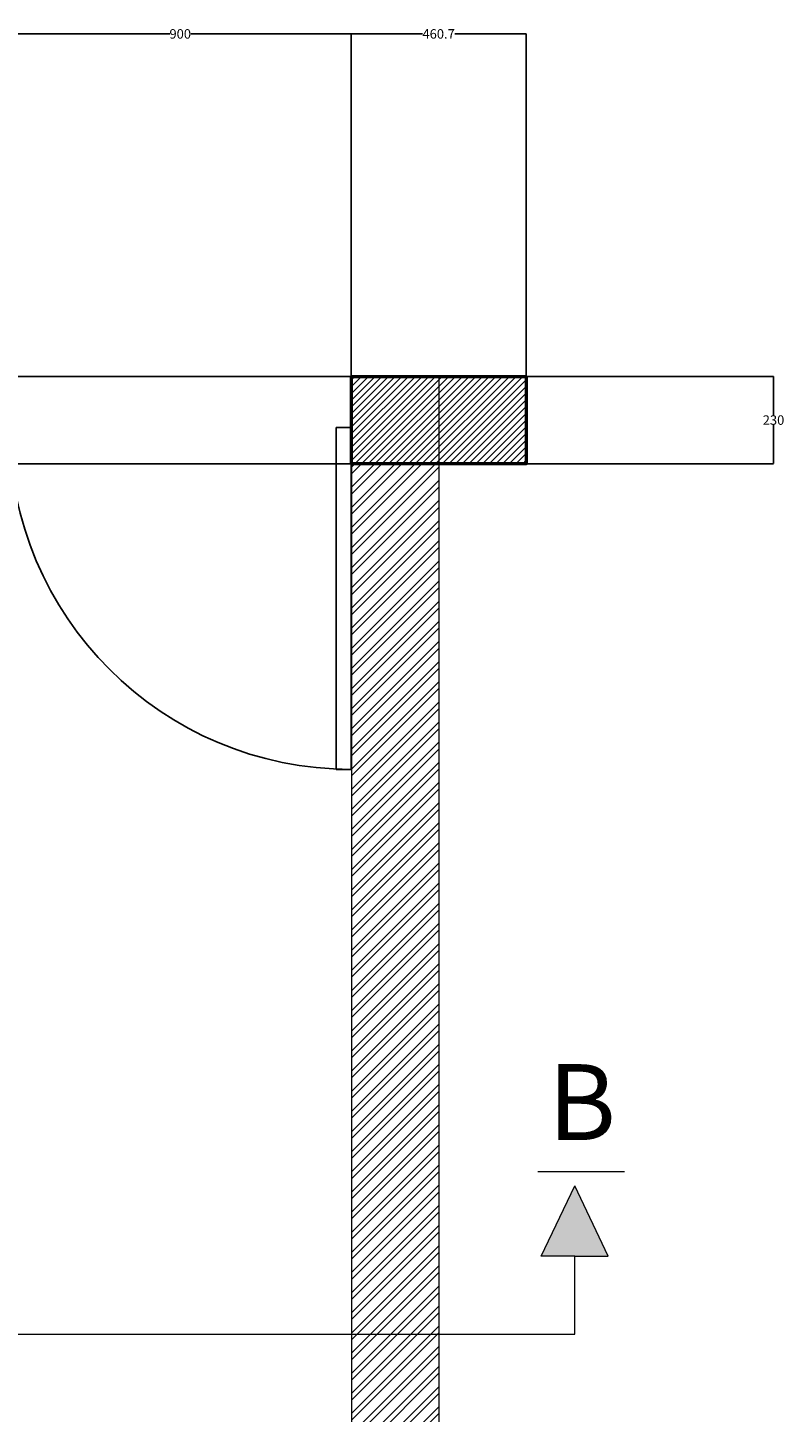
# Model space of a CAD drawing. Units: millimetres. Extents: x 1944 to 29915, y -10550 to 5909.
# Tile 9 of 24: x 9044 to 11036, y 2263 to 5909. Entities that reach past the tile are written whole.
import ezdxf

# ---------------------------------------------------------------- set-up
doc = ezdxf.new("R2010")
doc.units = ezdxf.units.MM
doc.header["$MEASUREMENT"] = 0
for name, color, linetype, lineweight in [('A-ANNO-DIMS', 2, 'Continuous', 18), ('A-ANNO-SYMB', 2, 'Continuous', 18), ('A-ANNO-TEXT', 7, 'Continuous', 25), ('A-DOOR', 4, 'Continuous', 25), ('A-FLOR-FIXT', 9, 'Continuous', 18), ('A-WALL', 7, 'Continuous', 50), ('A-WALL-PATT', 8, 'Continuous', 18)]:
    doc.layers.add(name, color=color, linetype=linetype, lineweight=lineweight)
doc.styles.get("Standard").update_dxf_attribs({"font": 'arial.ttf'})
doc.dimstyles.get("Standard").update_dxf_attribs({"dimtxt": 25, "dimasz": 0.18, "dimexe": 0.18, "dimexo": 0.0625, "dimgap": 0.09, "dimtad": 0, "dimtih": 1, "dimtoh": 1, "dimdec": 0, "dimzin": 0, "dimdsep": 46, "dimtxsty": 'Standard', "dimcen": 0.09, "dimadec": 0, "dimazin": 0, "dimtfac": 1, "dimtdec": 0, "dimtofl": 0, "dimtmove": 0, "dimatfit": 3, "dimfxl": 1, "dimtolj": 1, "dimtzin": 0, "dimarcsym": 0})

# ---------------------------------------------------------------- blocks, each defined once
blk = doc.blocks.new('*U2')
for p, q in [((0, 0), (0, -6)), ((40, 0), (40, -6))]:
    blk.add_line(p, q)
blk.add_lwpolyline([(0, 0), (0, 40), (1.75, 40), (1.75, 0)], close=True)
blk.add_arc((0, 0), 40, 0, 90)
blk = doc.blocks.new('*D47')
at = {"layer": 'A-ANNO-DIMS', "color": 0, "lineweight": -2, "transparency": 16777216}
for p, q in [((8995.2, 4990.9), (8995.2, 5892.9)), ((8995.4, 5892.8), (9417.6, 5892.8)), ((9895, 5892.8), (9472.9, 5892.8)), ((9895.2, 4990.9), (9895.2, 5892.9))]:
    blk.add_line(p, q, dxfattribs=at)
at = {"layer": 'A-ANNO-DIMS', "color": 0, "transparency": 16777216}
for points in [[(8995.4, 5892.8), (8995.4, 5892.7), (8995.2, 5892.8)], [(9895, 5892.8), (9895, 5892.7), (9895.2, 5892.8)]]:
    blk.add_solid(points, dxfattribs=at)
at = {"layer": 'Defpoints', "color": 0, "transparency": 16777216}
for p in [(9895.2, 5892.8), (8995.2, 4990.8), (9895.2, 4990.8)]:
    blk.add_point(p, dxfattribs=at)
at = {"layer": 'A-ANNO-DIMS', "color": 0, "transparency": 16777216, "insert": (9445.2, 5892.8), "char_height": 25, "attachment_point": 5}
blk.add_mtext('\\A1;900', dxfattribs=at)
blk = doc.blocks.new('*D48')
at = {"layer": 'A-ANNO-DIMS', "color": 0, "lineweight": -2, "transparency": 16777216}
for p, q in [((9895.2, 4990.9), (9895.2, 5892.9)), ((9895.4, 5892.8), (10082.8, 5892.8)), ((10355.8, 5892.8), (10168.4, 5892.8)), ((10355.9, 4990.9), (10355.9, 5892.9))]:
    blk.add_line(p, q, dxfattribs=at)
at = {"layer": 'A-ANNO-DIMS', "color": 0, "transparency": 16777216}
for points in [[(9895.4, 5892.8), (9895.4, 5892.7), (9895.2, 5892.8)], [(10355.8, 5892.8), (10355.8, 5892.7), (10355.9, 5892.8)]]:
    blk.add_solid(points, dxfattribs=at)
at = {"layer": 'Defpoints', "color": 0, "transparency": 16777216}
for p in [(10355.9, 5892.8), (9895.2, 4990.8), (10355.9, 4990.8)]:
    blk.add_point(p, dxfattribs=at)
at = {"layer": 'A-ANNO-DIMS', "color": 0, "transparency": 16777216, "insert": (10125.6, 5892.8), "char_height": 25, "attachment_point": 5}
blk.add_mtext('\\A1;460.7', dxfattribs=at)
blk = doc.blocks.new('*D55')
at = {"layer": 'A-ANNO-DIMS', "color": 0, "lineweight": -2, "transparency": 16777216}
for p, q in [((8995.3, 4990.8), (11007.7, 4990.8)), ((11007.5, 4990.7), (11007.5, 4888.7)), ((11007.5, 4761), (11007.5, 4863)), ((8995.3, 4760.8), (11007.7, 4760.8))]:
    blk.add_line(p, q, dxfattribs=at)
at = {"layer": 'A-ANNO-DIMS', "color": 0, "transparency": 16777216}
for points in [[(11007.5, 4990.7), (11007.5, 4990.7), (11007.5, 4990.8)], [(11007.5, 4761), (11007.5, 4761), (11007.5, 4760.8)]]:
    blk.add_solid(points, dxfattribs=at)
at = {"layer": 'Defpoints', "color": 0, "transparency": 16777216}
for p in [(8995.2, 4990.8), (8995.2, 4760.8), (11007.5, 4760.8)]:
    blk.add_point(p, dxfattribs=at)
at = {"layer": 'A-ANNO-DIMS', "color": 0, "transparency": 16777216, "insert": (11007.5, 4875.8), "char_height": 25, "attachment_point": 5}
blk.add_mtext('\\A1;230', dxfattribs=at)

msp = doc.modelspace()

# ---------------------------------------------------------------- hatches: boundary and pattern name
at = {"layer": 'A-ANNO-SYMB'}
h = msp.add_hatch(color=256, dxfattribs=at)
h.dxf.hatch_style = 1
h.paths.add_polyline_path([(10483.966, 2859.206), (10395.936, 2673.669), (10483.966, 2673.669), (10571.997, 2673.669)])
at = {"layer": 'A-WALL-PATT'}
h = msp.add_hatch(dxfattribs=at)
h.set_pattern_fill('ANSI31', color=256, scale=100)
h.paths.add_polyline_path([(9895.942, 4990.837), (9895.942, 4760.837), (10355.942, 4760.837), (10355.942, 4990.837)])
h = msp.add_hatch(dxfattribs=at)
h.set_pattern_fill('ANSI32', color=256, scale=100)
h.paths.add_polyline_path([(9895.942, 490.837), (10125.942, 490.837), (10125.942, 4760.837), (9895.942, 4760.837)])

# ---------------------------------------------------------------- linework, layer by layer
at = {"layer": 'A-ANNO-SYMB'}
for p, q in [((10571.997, 2673.669), (10483.966, 2859.206)), ((10483.966, 2468.085), (10483.966, 2673.669)), ((10483.966, 2673.669), (10571.997, 2673.669)), ((6293.436, 2468.085), (10483.966, 2468.085))]:
    msp.add_line(p, q, dxfattribs=at)
at = {"layer": 'A-DOOR'}
msp.add_line((8995.217, 4990.837), (9895.217, 4990.837), dxfattribs=at)
at = {"layer": 'A-FLOR-FIXT'}
for p, q in [((10386.764, 2896.746), (10615.254, 2896.746)), ((10395.936, 2673.669), (10483.966, 2859.206)), ((10483.966, 2673.669), (10395.936, 2673.669))]:
    msp.add_line(p, q, dxfattribs=at)
for points in [[(9895.942, 4990.837), (10125.942, 4990.837), (10125.942, 30.837), (9895.217, 30.837)], [(9895.942, 4760.837), (9895.942, 260.837), (9855.842, 260.837)]]:
    msp.add_lwpolyline(points, dxfattribs=at)
at = {"layer": 'A-WALL'}
msp.add_lwpolyline([(10355.942, 4990.837), (10355.942, 4760.837), (9895.942, 4760.837), (9895.942, 4990.837)], close=True, dxfattribs=at)

# ---------------------------------------------------------------- block references
at = {"layer": 'A-DOOR', "xscale": 22.5, "yscale": 22.5, "zscale": 22.5, "rotation": 180}
msp.add_blockref('*U2', (9895.217, 4855.837), dxfattribs=at)

# ---------------------------------------------------------------- texts
at = {"layer": 'A-ANNO-TEXT'}
msp.add_text('B', height=200, dxfattribs=at).set_placement((10413.511, 2979.554))

# ---------------------------------------------------------------- dimensions: what is measured, and where the dimension line sits
at = {"layer": 'A-ANNO-DIMS'}
for base, p1, p2, override, picture, middle in [((9895.217, 5892.769), (8995.217, 4990.837), (9895.217, 4990.837), {"dimdec": 0, "dimlfac": 1, "dimrnd": 0, "dimzin": 0, "dimdsep": 46, "dimlunit": 2}, '*D47', (9445.217, 5892.769)), ((10355.942, 5892.769), (9895.217, 4990.837), (10355.942, 4990.837), {"dimdec": 1, "dimlfac": 1, "dimrnd": 0, "dimzin": 0, "dimdsep": 46, "dimlunit": 2}, '*D48', (10125.58, 5892.769))]:
    dim = msp.add_linear_dim(base=base, p1=p1, p2=p2, dimstyle='Standard', override=override, dxfattribs=at)
    dim.commit()
    dim.dimension.update_dxf_attribs({"geometry": picture, "text_midpoint": middle})
dim = msp.add_linear_dim(base=(11007.504, 4760.837), p1=(8995.217, 4990.837), p2=(8995.217, 4760.837), angle=90, dimstyle='Standard', override={"dimdec": 0, "dimlfac": 1, "dimrnd": 0, "dimzin": 0, "dimdsep": 46, "dimlunit": 2}, dxfattribs=at)
dim.commit()
dim.dimension.update_dxf_attribs({"geometry": '*D55', "text_midpoint": (11007.504, 4875.837)})

doc.saveas('drawing.dxf')
